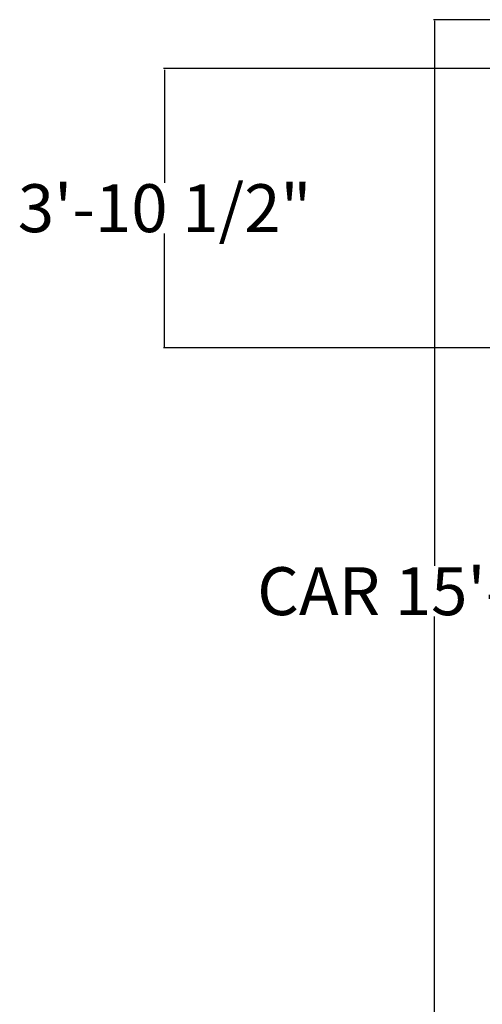
# Model space of a CAD drawing. Units: inches. Extents: x -4737294 to -4736756, y 1716389 to 1717040.
# Tile 6 of 25: x -4737294 to -4737217, y 1716491 to 1716656. Entities that reach past the tile are written whole.
import ezdxf

# ---------------------------------------------------------------- set-up
doc = ezdxf.new("R2010")
doc.units = ezdxf.units.IN
doc.header["$MEASUREMENT"] = 0
doc.layers.add('A-ANNO-DIMS', color=2, linetype='Continuous', lineweight=18)
doc.styles.get("Standard").update_dxf_attribs({"font": 'arial.ttf'})
doc.dimstyles.get("Standard").update_dxf_attribs({"dimtxt": 8, "dimasz": 0.18, "dimexe": 0.18, "dimexo": 0.0625, "dimgap": 0.09, "dimtad": 0, "dimtih": 1, "dimtoh": 1, "dimzin": 0, "dimdsep": 46, "dimlunit": 3, "dimtxsty": 'Standard', "dimcen": 0.09, "dimadec": 0, "dimazin": 0, "dimtfac": 1, "dimtofl": 0, "dimtmove": 0, "dimatfit": 3, "dimfxl": 1, "dimtolj": 1, "dimtzin": 0, "dimarcsym": 0})

# ---------------------------------------------------------------- blocks, each defined once
blk = doc.blocks.new('*D59')
at = {"layer": 'A-ANNO-DIMS', "color": 0, "lineweight": -2, "transparency": 16777216}
for p, q in [((-4737196.54, 1716655.66), (-4737225.28, 1716655.66)), ((-4737225.1, 1716655.48), (-4737225.1, 1716564.48)), ((-4737225.1, 1716465.02), (-4737225.1, 1716556.03)), ((-4737196.54, 1716464.84), (-4737225.28, 1716464.84))]:
    blk.add_line(p, q, dxfattribs=at)
at = {"layer": 'A-ANNO-DIMS', "color": 0, "transparency": 16777216}
for points in [[(-4737225.13, 1716655.48), (-4737225.07, 1716655.48), (-4737225.1, 1716655.66)], [(-4737225.13, 1716465.02), (-4737225.07, 1716465.02), (-4737225.1, 1716464.84)]]:
    blk.add_solid(points, dxfattribs=at)
at = {"layer": 'Defpoints', "color": 0, "transparency": 16777216}
for p in [(-4737196.48, 1716655.66), (-4737225.1, 1716464.84), (-4737196.48, 1716464.84)]:
    blk.add_point(p, dxfattribs=at)
at = {"layer": 'A-ANNO-DIMS', "color": 0, "transparency": 16777216, "insert": (-4737225.1, 1716560.25), "char_height": 8, "attachment_point": 5}
blk.add_mtext('\\A1;CAR 15\'-11"', dxfattribs=at)
blk = doc.blocks.new('*D63')
at = {"layer": 'A-ANNO-DIMS', "color": 0, "lineweight": -2, "transparency": 16777216}
for p, q in [((-4737062.21, 1716647.49), (-4737270.32, 1716647.49)), ((-4737270.14, 1716647.31), (-4737270.14, 1716628.42)), ((-4737270.14, 1716601.06), (-4737270.14, 1716619.96)), ((-4737062.21, 1716600.88), (-4737270.32, 1716600.88))]:
    blk.add_line(p, q, dxfattribs=at)
at = {"layer": 'A-ANNO-DIMS', "color": 0, "transparency": 16777216}
for points in [[(-4737270.17, 1716647.31), (-4737270.11, 1716647.31), (-4737270.14, 1716647.49)], [(-4737270.17, 1716601.06), (-4737270.11, 1716601.06), (-4737270.14, 1716600.88)]]:
    blk.add_solid(points, dxfattribs=at)
at = {"layer": 'Defpoints', "color": 0, "transparency": 16777216}
for p in [(-4737270.14, 1716647.49), (-4737062.14, 1716647.49), (-4737062.14, 1716600.88)]:
    blk.add_point(p, dxfattribs=at)
at = {"layer": 'A-ANNO-DIMS', "color": 0, "transparency": 16777216, "insert": (-4737270.14, 1716624.19), "char_height": 8, "attachment_point": 5}
blk.add_mtext('\\A1;3\'-10 1/2"', dxfattribs=at)

msp = doc.modelspace()

# ---------------------------------------------------------------- dimensions: what is measured, and where the dimension line sits
at = {"layer": 'A-ANNO-DIMS'}
dim = msp.add_linear_dim(base=(-4737225.099, 1716464.844), p1=(-4737196.476, 1716655.661), p2=(-4737196.476, 1716464.844), angle=270, text='CAR <>', dimstyle='Standard', override={"dimdec": 1, "dimlfac": 1, "dimrnd": 0, "dimzin": 1, "dimdsep": 46, "dimlunit": 4, "dimfrac": 2}, dxfattribs=at)
dim.commit()
dim.dimension.update_dxf_attribs({"geometry": '*D59', "text_midpoint": (-4737225.099, 1716560.253)})
dim = msp.add_linear_dim(base=(-4737270.144, 1716647.493), p1=(-4737062.144, 1716600.884), p2=(-4737062.144, 1716647.493), angle=90, dimstyle='Standard', override={"dimdec": 1, "dimlfac": 1, "dimrnd": 0, "dimzin": 1, "dimdsep": 46, "dimlunit": 4, "dimfrac": 2}, dxfattribs=at)
dim.commit()
dim.dimension.update_dxf_attribs({"geometry": '*D63', "text_midpoint": (-4737270.144, 1716624.188)})

doc.saveas('drawing.dxf')
